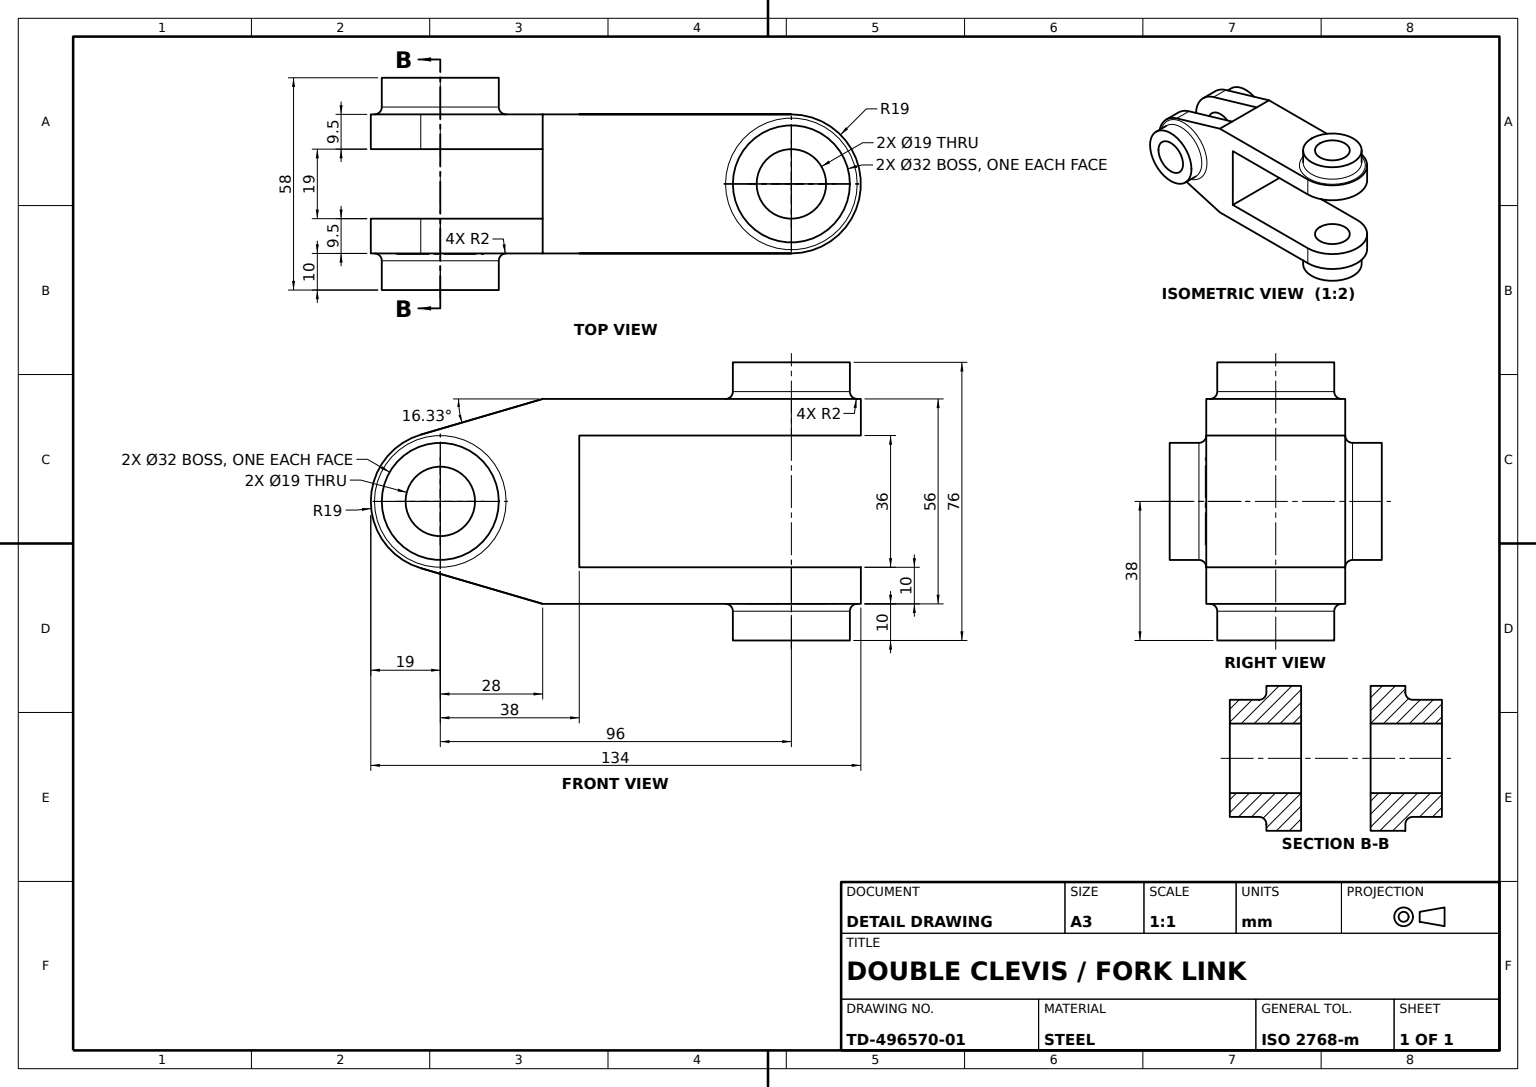
SolidWorks part; units mm, degrees
material "Plain Carbon Steel"
ref_plane "Front Plane" through (0, 0, 0) normal (0, 0, 1) x (1, 0, 0)
ref_plane "Top Plane" through (0, 0, 0) normal (0, 1, 0) x (1, 0, 0)
ref_plane "Right Plane" through (0, 0, 0) normal (1, 0, 0) x (0, 0, -1)
sketch "Link Body Profile Sketch" plane through (0, 0, 0) normal (0, 0, 1) x (1, 0, 0)
  line L0 (-5.341, 18.2339) -> (28, 28)
  line L1 (28, 28) -> (96, 28)
  line L2 (96, 28) -> (96, 18)
  line L3 (96, 18) -> (38, 18)
  line L4 (38, 18) -> (38, -18)
  line L5 (38, -18) -> (96, -18)
  line L6 (96, -18) -> (96, -28)
  line L7 (96, -28) -> (28, -28)
  line L8 (28, -28) -> (-5.341, -18.2339)
  line L9 (0, 0) -> (65.6057, 0) construction
  arc A0 (-5.341, 18.2339) -> (-5.341, -18.2339) centre (0, 0) ccw
  circle A1 centre (0, 0) radius 9.5
  dimension "D1" = 38
  dimension "D2" = 19
  dimension "D3" = 28
  dimension "D4" = 38
  dimension "D5" = 10
  dimension "D6" = 56
  dimension "D7" = 96
extrude "Link Body 38mm" add sketch "Link Body Profile Sketch" along normal mid plane 38
sketch "Fork End Boss A Sketch" plane through (0, 28, 0) normal (0, 1, 0) x (1, 0, 0)
  line L0 (96, -19) -> (96, 19) construction
  circle A0 centre (96, 0) radius 19
extrude "Fork End Boss A" add sketch "Fork End Boss A Sketch" against normal up to surface (10 mm away) up to face at (67, 18, 0)
sketch "Fork End Boss B Sketch" plane through (0, -28, 0) normal (0, -1, 0) x (1, 0, 0)
  line L0 (96, 19) -> (96, -19) construction
  circle A0 centre (96, 0) radius 19
  arc A1 (96, -19) -> (96, 19) centre (96, 0) ccw construction
extrude "Fork End Boss B" add sketch "Fork End Boss B Sketch" against normal up to surface (10 mm away) up to face at (67, -18, 0)
sketch "Fork Slot Sketch" plane through (0, -28, 0) normal (0, -1, 0) x (1, 0, 0)
  line L0 (-19, 19) -> (-19, -19) construction
  line L1 (-19, 9.5) -> (28, 9.5)
  line L2 (-19, 9.5) -> (-19, -9.5)
  line L3 (-19, -9.5) -> (28, -9.5)
  line L4 (28, 9.5) -> (28, -9.5)
  line L5 (28, 19) -> (28, -19) construction
  line L7 (28, 19) -> (28, -19) construction
  point P8 (28, 0)
  point P9 (28, 0)
  dimension "D1" = 19
extrude "Fork Slot 19mm" cut sketch "Fork Slot Sketch" against normal blind 67
sketch "Side Hub Sketch Ø32" plane through (0, 0, 19) normal (0, 0, 1) x (1, 0, 0)
  circle A0 centre (0, 0) radius 16
  circle A1 centre (0, 0) radius 9.5 construction
  circle A2 centre (0, 0) radius 9.5
  dimension "D1" = 32
extrude "Side Hub Ø32" add sketch "Side Hub Sketch Ø32" along normal blind 10
mirror "Side Hub Mirror" about plane through (0, 0, 0) normal (0, 0, 1) of "Side Hub Ø32"
sketch "Fork Hub Sketch Ø32" plane through (0, 28, 0) normal (0, 1, 0) x (1, 0, 0)
  circle A0 centre (96, 0) radius 16
  arc A1 (96, -19) -> (96, 19) centre (96, 0) ccw construction
  dimension "D1" = 32
extrude "Fork Hub Ø32" add sketch "Fork Hub Sketch Ø32" along normal blind 10
mirror "Fork Hub Mirror" about plane through (0, 0, 0) normal (0, 1, 0) of "Fork Hub Ø32"
sketch "Fork Pin Bore Sketch Ø19" plane through (0, -38, 0) normal (0, -1, 0) x (1, 0, 0)
  circle A0 centre (96, 0) radius 9.5
  circle A1 centre (96, 0) radius 16 construction
  dimension "D1" = 19
extrude "Fork Pin Bore Ø19" cut sketch "Fork Pin Bore Sketch Ø19" against normal through all
fillet "Edge Fillets R2" radius 2 4 edges at (80, -28, 0) (112, 28, 0) (16, 0, -19) (16, 0, 19)
